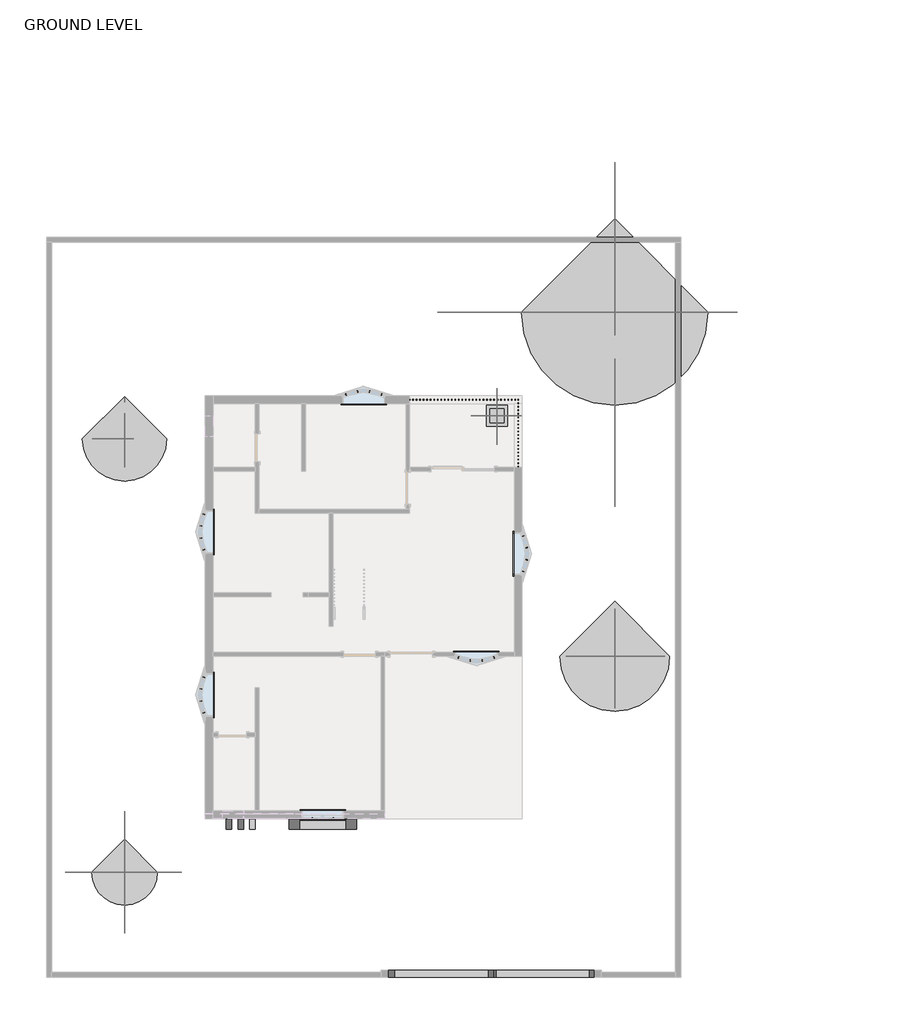
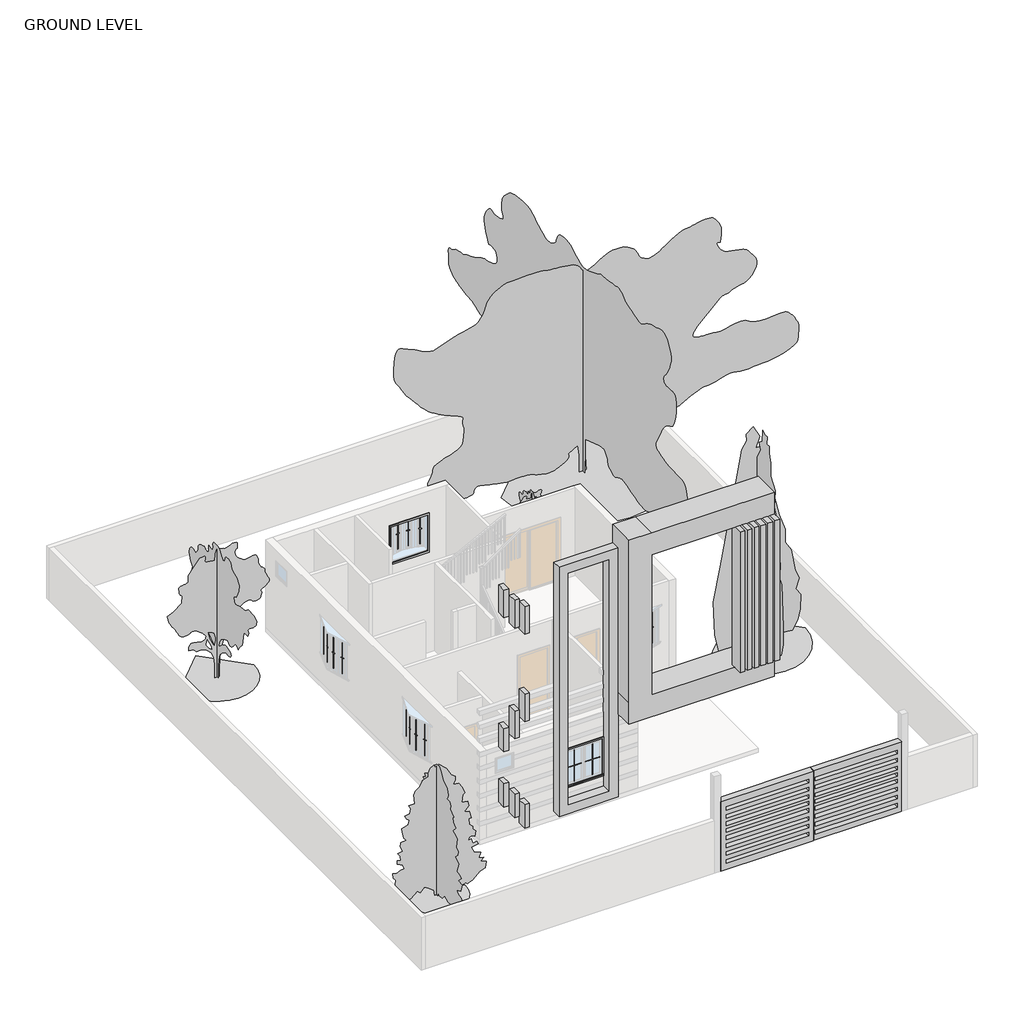
# One storey, part 3 of 3: 30 proxies, 6 geographic elements, 1 railing.
# Revit data of these elements (continued)
# Element 30 (IfcBuildingElementProxy, "Trim-Window-Interior-Flat : Picture Frame") (continued)
#   Materials on its faces: "Wood - Stained"
# Element 31 (IfcGeographicElement, "Planter : 2'x2'")
#   Phase Created = New Construction
#   Materials on its faces: "Concrete, Precast"
# Element 32 (IfcGeographicElement, "RPC Tree - Conifer")
#   Phase Created = New Construction
# Element 33 (IfcGeographicElement, "RPC Tree - Conifer : Red Cedar - 10' 2")
#   Phase Created = New Construction
# Element 34 (IfcGeographicElement, "RPC Tree - Deciduous : 15'")
#   Phase Created = New Construction
# Element 35 (IfcGeographicElement, "RPC Tree - Deciduous : Japanese Cherry - 15'")
#   Phase Created = New Construction
# Element 36 (IfcGeographicElement, "RPC Tree - Deciduous : Japanese Cherry - 15' 2")
#   Phase Created = New Construction
# Element 37 (IfcRailing, "Handrail - Rectangular")
#   built-in parameter 1008621 = 2 (stored number, unit not read)
#   Phase Created = New Construction
# Materials
#   "Concrete, Precast": class "Concrete", colour RGB 198 187 187, transparency 0, Description = "Precast concrete", Cost = 0
#   "wall 1": class "Generic", colour RGB 67 39 34, transparency 0, Cost = 0
#   "Copper": class "Metal", colour RGB 0 0 0, transparency 0, Description = "Copper, matte finish", Cost = 0
#   "Wood Planks": class "Wood", colour RGB 193 160 115, transparency 0, Description = "Physical material.", Cost = 0
#   "wall": class "Generic", colour RGB 86 92 74, transparency 0, Cost = 0
#   "Clad - White": class "Wood", colour RGB 242 242 238, transparency 0, Cost = 0
#   "Wood - Stained": class "Wood", colour RGB 224 178 126, transparency 0, Cost = 0
